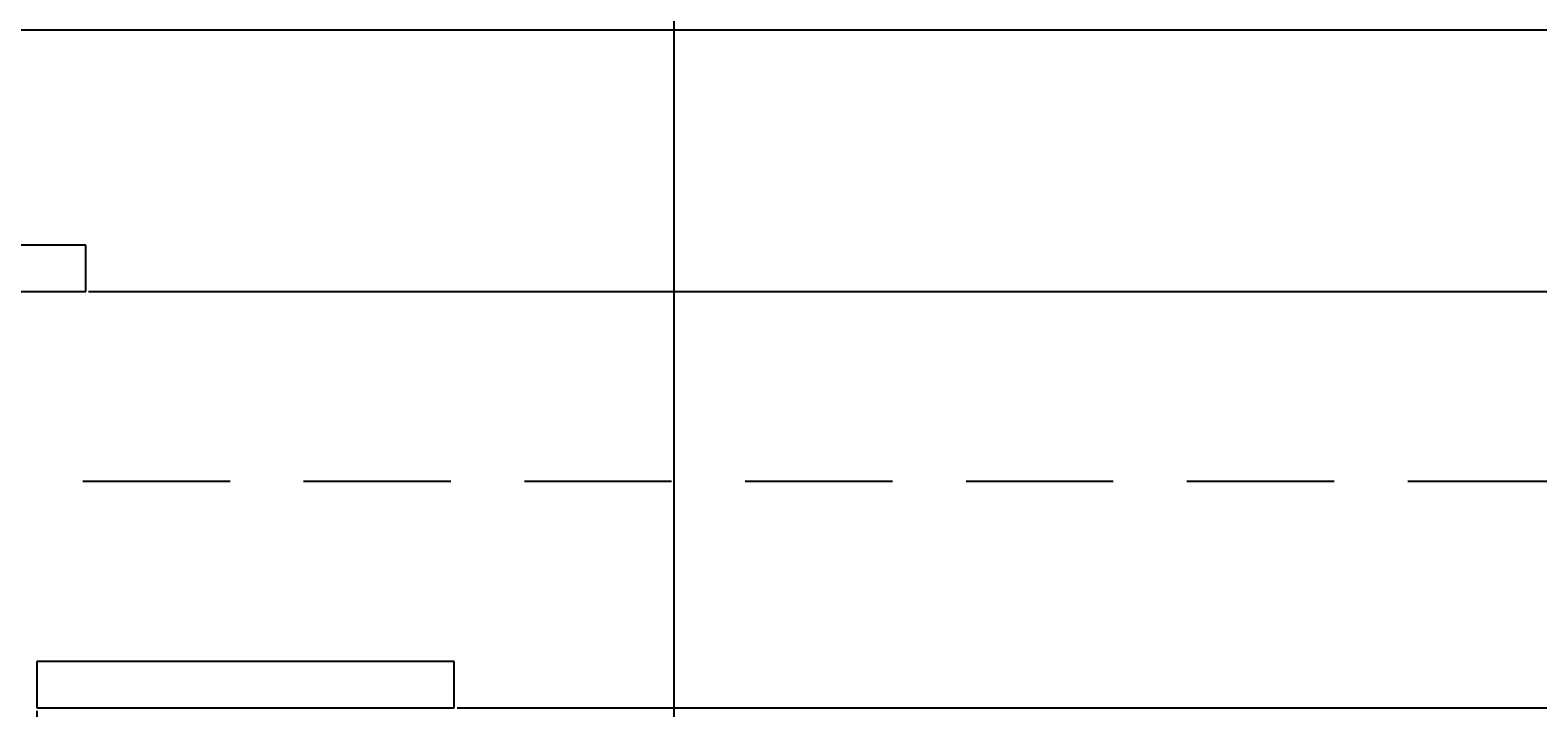
# Model space of a CAD drawing. Units: inches. Extents: x 2812 to 3051, y 1398 to 1659.
# Tile 18 of 65: x 2897 to 2929, y 1457 to 1472. Entities that reach past the tile are written whole.
import ezdxf

# ---------------------------------------------------------------- set-up
doc = ezdxf.new("R2010")
doc.units = ezdxf.units.IN
doc.linetypes.add('HIDDEN2', pattern=[4.7625, 3.175, -1.5875])
for name, color, linetype, lineweight in [('A-ANNO-DIMS', 2, 'Continuous', 18), ('S-CONC-HIDN', 8, 'HIDDEN2', 25), ('S-STEP', 3, 'Continuous', 25)]:
    doc.layers.add(name, color=color, linetype=linetype, lineweight=lineweight)
doc.styles.get("Standard").update_dxf_attribs({"font": 'arial.ttf'})
doc.dimstyles.get("Standard").update_dxf_attribs({"dimtxt": 0.18, "dimasz": 0.18, "dimexe": 0.18, "dimexo": 0.0625, "dimgap": 0.09, "dimtad": 0, "dimtih": 1, "dimtoh": 1, "dimdec": 4, "dimzin": 0, "dimdsep": 46, "dimtxsty": 'Standard', "dimcen": 0.09, "dimadec": 0, "dimazin": 0, "dimtfac": 1, "dimtdec": 4, "dimtofl": 0, "dimtmove": 0, "dimatfit": 3, "dimfxl": 1, "dimtolj": 1, "dimtzin": 0, "dimarcsym": 0})

# ---------------------------------------------------------------- blocks, each defined once
blk = doc.blocks.new('STEP-IRON-4')
for p, q in [((9, 1), (0, 1)), ((0, 1), (0, 0)), ((9, 0), (9, 1)), ((0, 0), (9, 0)), ((0, 0), (5.792, 0))]:
    blk.add_line(p, q)
blk = doc.blocks.new('STEP-IRON-5')
for p, q in [((9, 1), (0, 1)), ((0, 1), (0, 0)), ((9, 0), (9, 1)), ((0, 0), (9, 0))]:
    blk.add_line(p, q)
blk = doc.blocks.new('*D29')
at = {"layer": 'A-ANNO-DIMS', "color": 0, "lineweight": -2, "transparency": 16777216}
for p, q in [((2910.742, 1598.757), (2910.742, 1397.505)), ((2883.385, 1559.757), (2883.385, 1397.505)), ((2883.565, 1397.685), (2896.598, 1397.685)), ((2910.562, 1397.685), (2897.528, 1397.685))]:
    blk.add_line(p, q, dxfattribs=at)
at = {"layer": 'A-ANNO-DIMS', "color": 0, "transparency": 16777216}
for points in [[(2883.565, 1397.715), (2883.565, 1397.655), (2883.385, 1397.685)], [(2910.562, 1397.715), (2910.562, 1397.655), (2910.742, 1397.685)]]:
    blk.add_solid(points, dxfattribs=at)
at = {"layer": 'Defpoints', "color": 0, "transparency": 16777216}
for p in [(2910.742, 1598.82), (2883.385, 1559.82), (2910.742, 1397.685)]:
    blk.add_point(p, dxfattribs=at)
at = {"layer": 'A-ANNO-DIMS', "color": 0, "transparency": 16777216, "insert": (2897.063, 1397.685), "char_height": 0.18, "attachment_point": 5}
blk.add_mtext('\\A1;27.357', dxfattribs=at)
blk = doc.blocks.new('*D45')
at = {"layer": 'A-ANNO-DIMS', "color": 0, "lineweight": -2, "transparency": 16777216}
for p, q in [((2896.385, 1487.973), (2896.385, 1397.505)), ((2941.385, 1487.973), (2941.385, 1397.505)), ((2896.565, 1397.685), (2918.662, 1397.685)), ((2941.205, 1397.685), (2919.108, 1397.685))]:
    blk.add_line(p, q, dxfattribs=at)
at = {"layer": 'A-ANNO-DIMS', "color": 0, "transparency": 16777216}
for points in [[(2896.565, 1397.715), (2896.565, 1397.655), (2896.385, 1397.685)], [(2941.205, 1397.715), (2941.205, 1397.655), (2941.385, 1397.685)]]:
    blk.add_solid(points, dxfattribs=at)
at = {"layer": 'Defpoints', "color": 0, "transparency": 16777216}
for p in [(2896.385, 1488.035), (2941.385, 1488.035), (2941.385, 1397.685)]:
    blk.add_point(p, dxfattribs=at)
at = {"layer": 'A-ANNO-DIMS', "color": 0, "transparency": 16777216, "insert": (2918.885, 1397.685), "char_height": 0.18, "attachment_point": 5}
blk.add_mtext('\\A1;45', dxfattribs=at)
blk = doc.blocks.new('*D60')
at = {"layer": 'A-ANNO-DIMS', "color": 0, "lineweight": -2, "transparency": 16777216}
for p, q in [((2889.058, 1466.34), (2889.058, 1397.505)), ((2897.002, 1457.364), (2897.002, 1397.505)), ((2889.238, 1397.685), (2892.637, 1397.685)), ((2896.822, 1397.685), (2893.422, 1397.685))]:
    blk.add_line(p, q, dxfattribs=at)
at = {"layer": 'A-ANNO-DIMS', "color": 0, "transparency": 16777216}
for points in [[(2889.238, 1397.715), (2889.238, 1397.655), (2889.058, 1397.685)], [(2896.822, 1397.715), (2896.822, 1397.655), (2897.002, 1397.685)]]:
    blk.add_solid(points, dxfattribs=at)
at = {"layer": 'Defpoints', "color": 0, "transparency": 16777216}
for p in [(2889.058, 1466.402), (2897.002, 1457.426), (2897.002, 1397.685)]:
    blk.add_point(p, dxfattribs=at)
at = {"layer": 'A-ANNO-DIMS', "color": 0, "transparency": 16777216, "insert": (2893.03, 1397.685), "char_height": 0.18, "attachment_point": 5}
blk.add_mtext('\\A1;7.944', dxfattribs=at)
blk = doc.blocks.new('*D68')
at = {"layer": 'A-ANNO-DIMS', "color": 0, "lineweight": -2, "transparency": 16777216}
for p, q in [((2898.12, 1466.402), (3051.178, 1466.402)), ((3050.998, 1466.222), (3050.998, 1462.096)), ((3050.998, 1457.606), (3050.998, 1461.733)), ((2906.065, 1457.426), (3051.178, 1457.426))]:
    blk.add_line(p, q, dxfattribs=at)
at = {"layer": 'A-ANNO-DIMS', "color": 0, "transparency": 16777216}
for points in [[(3050.968, 1466.222), (3051.028, 1466.222), (3050.998, 1466.402)], [(3050.968, 1457.606), (3051.028, 1457.606), (3050.998, 1457.426)]]:
    blk.add_solid(points, dxfattribs=at)
at = {"layer": 'Defpoints', "color": 0, "transparency": 16777216}
for p in [(2898.058, 1466.402), (3050.998, 1466.402), (2906.002, 1457.426)]:
    blk.add_point(p, dxfattribs=at)
at = {"layer": 'A-ANNO-DIMS', "color": 0, "transparency": 16777216, "insert": (3050.998, 1461.914), "char_height": 0.18, "attachment_point": 5}
blk.add_mtext('\\A1;8.976', dxfattribs=at)
blk = doc.blocks.new('*D77')
at = {"layer": 'A-ANNO-DIMS', "color": 0, "lineweight": -2, "transparency": 16777216}
for p, q in [((2961.322, 1472.035), (2811.806, 1472.035)), ((2811.986, 1471.855), (2811.986, 1461.436)), ((2811.986, 1450.654), (2811.986, 1461.073)), ((2963.812, 1450.474), (2811.806, 1450.474))]:
    blk.add_line(p, q, dxfattribs=at)
at = {"layer": 'A-ANNO-DIMS', "color": 0, "transparency": 16777216}
for points in [[(2811.956, 1471.855), (2812.016, 1471.855), (2811.986, 1472.035)], [(2811.956, 1450.654), (2812.016, 1450.654), (2811.986, 1450.474)]]:
    blk.add_solid(points, dxfattribs=at)
at = {"layer": 'Defpoints', "color": 0, "transparency": 16777216}
for p in [(2811.986, 1472.035), (2961.385, 1472.035), (2963.874, 1450.474)]:
    blk.add_point(p, dxfattribs=at)
at = {"layer": 'A-ANNO-DIMS', "color": 0, "transparency": 16777216, "insert": (2811.986, 1461.255), "char_height": 0.18, "attachment_point": 5}
blk.add_mtext('\\A1;21.56', dxfattribs=at)

msp = doc.modelspace()

# ---------------------------------------------------------------- linework, layer by layer
at = {"layer": 'S-CONC-HIDN'}
msp.add_line((3029.7562, 1462.3026), (2835.3849, 1462.3026), dxfattribs=at)

# ---------------------------------------------------------------- block references
at = {"layer": 'S-STEP'}
for name, p in [('STEP-IRON-5', (2889.0578, 1466.402)), ('STEP-IRON-4', (2897.0023, 1457.4261))]:
    msp.add_blockref(name, p, dxfattribs=at)

# ---------------------------------------------------------------- dimensions: what is measured, and where the dimension line sits
at = {"layer": 'A-ANNO-DIMS'}
for base, p1, p2, override, picture, middle in [((2910.7415, 1397.6854), (2883.3849, 1559.82), (2910.7415, 1598.82), {"dimdec": 3, "dimlfac": 1, "dimrnd": 0, "dimzin": 0, "dimdsep": 46, "dimlunit": 2}, '*D29', (2897.0632, 1397.6854)), ((2941.3849, 1397.6854), (2896.3849, 1488.0354), (2941.3849, 1488.0354), {"dimdec": 0, "dimlfac": 1, "dimrnd": 0, "dimzin": 0, "dimdsep": 46, "dimlunit": 2}, '*D45', (2918.8849, 1397.6854)), ((2897.0021, 1397.6854), (2889.0577, 1466.4024), (2897.0021, 1457.4265), {"dimdec": 3, "dimlfac": 1, "dimrnd": 0, "dimzin": 0, "dimdsep": 46, "dimlunit": 2}, '*D60', (2893.0299, 1397.6854))]:
    dim = msp.add_linear_dim(base=base, p1=p1, p2=p2, dimstyle='Standard', override=override, dxfattribs=at)
    dim.commit()
    dim.dimension.update_dxf_attribs({"geometry": picture, "text_midpoint": middle})
for base, p1, p2, override, picture, middle in [((2811.9855, 1472.0354), (2963.8741, 1450.4738), (2961.3849, 1472.0354), {"dimdec": 2, "dimlfac": 1, "dimrnd": 0, "dimzin": 0, "dimdsep": 46, "dimlunit": 2}, '*D77', (2811.9855, 1461.2546)), ((3050.998, 1466.4024), (2906.0021, 1457.4265), (2898.0577, 1466.4024), {"dimdec": 3, "dimlfac": 1, "dimrnd": 0, "dimzin": 0, "dimdsep": 46, "dimlunit": 2}, '*D68', (3050.998, 1461.9144))]:
    dim = msp.add_linear_dim(base=base, p1=p1, p2=p2, angle=90, dimstyle='Standard', override=override, dxfattribs=at)
    dim.commit()
    dim.dimension.update_dxf_attribs({"geometry": picture, "text_midpoint": middle})

doc.saveas('drawing.dxf')
